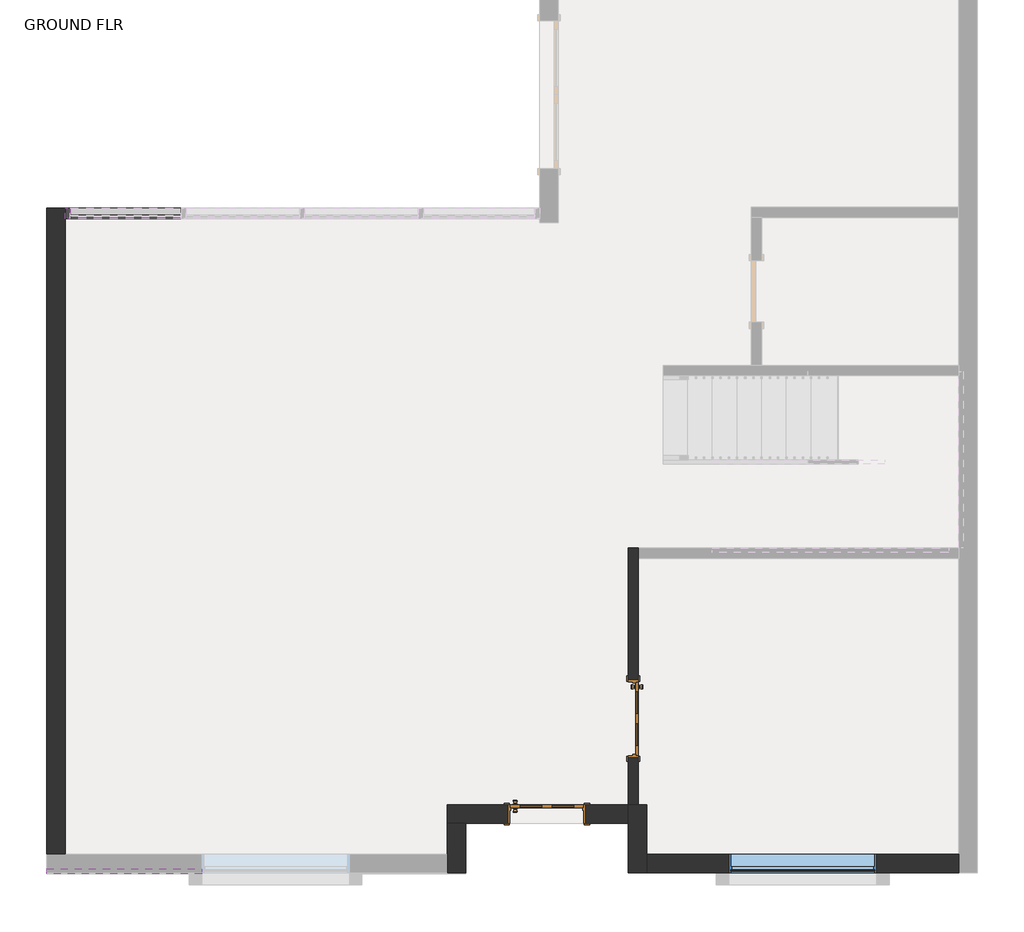
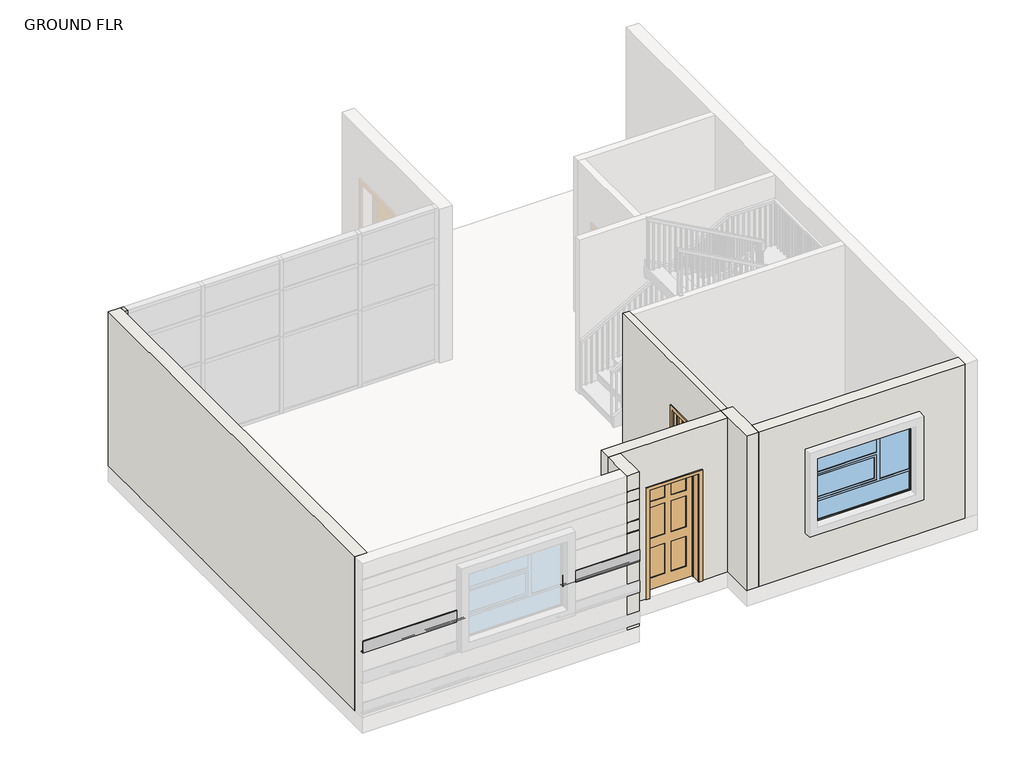
# One storey, part 2 of 4: 6 walls, 4 members, 2 doors, 1 proxy, 1 window.
"""IFC4 building model written with IfcOpenShell, lengths in millimetres."""

from ifc_helpers import new_model, si_unit, point, frame, frame_2d, origin, place, context, project, spatial, polyline, circle_curve, trimmed, segment, composite_curve, outline, extrude, faceted_brep, transform, mapped, element, save
from ifc_brep_helpers import plane_surface, cylinder_surface, revolved_surface, advanced_brep
from components import door_03e3dfb5, door_d86b6c54, member_bb3ab01a, member_47bfaf8a, member_4491d118, member_73c23c35, window_dd9b4f56

model = new_model("IFC4")

# Units and contexts
model_context = context("Model", 3, world=origin())
ifc_project = project(units=[si_unit("LENGTHUNIT", "METRE", prefix="MILLI")], contexts=[model_context])

# Site, building, storey
site = spatial("IfcSite", under=ifc_project)
building = spatial("IfcBuilding", under=site)
storey = spatial("IfcBuildingStorey", under=building, Name="GROUND FLR", Elevation=304.8)

# Proxy
placement = place(None, origin())
element("IfcBuildingElementProxy", 1, Name="Reveal", ObjectType="Reveal", at=placement, inside=storey, context=model_context, shape_type="SweptSolid", body=[
    extrude(outline(composite_curve([segment(polyline([(-2464.7620789, 1824.113469), (-2401.5160789, 1824.113469), (-2401.5160789, 1822.7337932)]), True, "CONTINUOUS"), segment(trimmed(circle_curve(frame_2d((-2406.7611789, 1822.7337932)), 5.2451), [point((-2401.5160789, 1822.7337932))], [point((-2405.8988881, 1817.5600587))], False, "CARTESIAN"), True, "CONTINUOUS"), segment(polyline([(-2405.8988881, 1817.5600587), (-2429.5195789, 1813.623269), (-2448.7574605, 1810.416949)]), True, "CONTINUOUS"), segment(trimmed(circle_curve(frame_2d((-2447.0328789, 1800.06948)), 10.4902), [point((-2448.7574605, 1810.416949))], [point((-2457.5230789, 1800.06948))], True, "CARTESIAN"), True, "CONTINUOUS"), segment(polyline([(-2457.5230789, 1800.06948), (-2457.5230789, 1619.557458)]), True, "CONTINUOUS"), segment(trimmed(circle_curve(frame_2d((-2447.0328789, 1619.557458)), 10.4902), [point((-2457.5230789, 1619.557458))], [point((-2448.7574605, 1609.209989))], True, "CARTESIAN"), True, "CONTINUOUS"), segment(polyline([(-2448.7574605, 1609.209989), (-2429.5195789, 1606.003669), (-2405.8988881, 1602.0668793)]), True, "CONTINUOUS"), segment(trimmed(circle_curve(frame_2d((-2406.7611789, 1596.8931449)), 5.2451), [point((-2405.8988881, 1602.0668793))], [point((-2401.5160789, 1596.8931449))], False, "CARTESIAN"), True, "CONTINUOUS"), segment(polyline([(-2401.5160789, 1596.8931449), (-2401.5160789, 1595.513469), (-2464.7620789, 1595.513469), (-2464.7620789, 1824.113469)]), True, "CONTINUOUS")], self_intersect=False)), frame((-2097.5328791, 0.0, 0.0), z_axis=(1.0, 0.0, 0.0), x_axis=(0.0, 1.0, 0.0)), (0.0, 0.0, 1.0), 1435.1),
    extrude(outline(composite_curve([segment(polyline([(-2464.7620789, 1824.113469), (-2401.5160789, 1824.113469), (-2401.5160789, 1822.7337932)]), True, "CONTINUOUS"), segment(trimmed(circle_curve(frame_2d((-2406.7611789, 1822.7337932)), 5.2451), [point((-2401.5160789, 1822.7337932))], [point((-2405.8988881, 1817.5600587))], False, "CARTESIAN"), True, "CONTINUOUS"), segment(polyline([(-2405.8988881, 1817.5600587), (-2429.5195789, 1813.623269), (-2448.7574605, 1810.416949)]), True, "CONTINUOUS"), segment(trimmed(circle_curve(frame_2d((-2447.0328789, 1800.06948)), 10.4902), [point((-2448.7574605, 1810.416949))], [point((-2457.5230789, 1800.06948))], True, "CARTESIAN"), True, "CONTINUOUS"), segment(polyline([(-2457.5230789, 1800.06948), (-2457.5230789, 1619.557458)]), True, "CONTINUOUS"), segment(trimmed(circle_curve(frame_2d((-2447.0328789, 1619.557458)), 10.4902), [point((-2457.5230789, 1619.557458))], [point((-2448.7574605, 1609.209989))], True, "CARTESIAN"), True, "CONTINUOUS"), segment(polyline([(-2448.7574605, 1609.209989), (-2429.5195789, 1606.003669), (-2405.8988881, 1602.0668793)]), True, "CONTINUOUS"), segment(trimmed(circle_curve(frame_2d((-2406.7611789, 1596.8931449)), 5.2451), [point((-2405.8988881, 1602.0668793))], [point((-2401.5160789, 1596.8931449))], False, "CARTESIAN"), True, "CONTINUOUS"), segment(polyline([(-2401.5160789, 1596.8931449), (-2401.5160789, 1595.513469), (-2464.7620789, 1595.513469), (-2464.7620789, 1824.113469)]), True, "CONTINUOUS")], self_intersect=False)), frame((-5844.0328791, 0.0, 0.0), z_axis=(1.0, 0.0, 0.0), x_axis=(0.0, 1.0, 0.0)), (0.0, 0.0, 1.0), 1917.7),
])

# Doors
door_shape = door_03e3dfb5(model_context)
element("IfcDoor", 2, ObjectType="Door-Interior-Single-6_Panel-Wood : 36\" x 84\"", at=placement, inside=storey, context=model_context, shape_type="MappedRepresentation", body=[
    mapped(door_shape, transform((1410.8421209, -544.8776789, 304.8), x_axis=(0.0, -1.0, 0.0), y_axis=(1.0, 0.0, 0.0), z_axis=(0.0, 0.0, 1.0))),
])
door_2_shape = door_d86b6c54(model_context)
element("IfcDoor", 3, ObjectType="Door-Interior-Single-6_Panel-Wood : 36\" x 84\"", at=placement, inside=storey, context=model_context, shape_type="MappedRepresentation", body=[
    mapped(door_2_shape, transform((340.8671209, -1722.8026789, 304.8), x_axis=(1.0, 0.0, 0.0), y_axis=(0.0, 1.0, 0.0), z_axis=(0.0, 0.0, 1.0))),
])

# Members
member_shape = member_bb3ab01a(model_context)
element("IfcMember", 4, ObjectType="Rectangular Mullion : 2.5\" x 5\" rectangular", at=placement, inside=storey, context=model_context, shape_type="MappedRepresentation", body=[
    mapped(member_shape, transform((-5551.9328791, 5703.5223211, 304.8), x_axis=(0.0, 0.0, -1.0), y_axis=(0.0, -1.0, 0.0), z_axis=(-1.0, 0.0, 0.0))),
])
member_2_shape = member_47bfaf8a(model_context)
element("IfcMember", 5, ObjectType="Rectangular Mullion : 2.5\" x 5\" rectangular", at=placement, inside=storey, context=model_context, shape_type="MappedRepresentation", body=[
    mapped(member_2_shape, transform((-5615.4328791, 5703.5223211, 3352.8), x_axis=(-1.0, 0.0, 0.0), y_axis=(0.0, -1.0, 0.0), z_axis=(0.0, 0.0, 1.0))),
])
member_3_shape = member_4491d118(model_context)
element("IfcMember", 6, ObjectType="Rectangular Mullion : 2.5\" x 5\" rectangular", at=placement, inside=storey, context=model_context, shape_type="MappedRepresentation", body=[
    mapped(member_3_shape, transform((-5615.4328791, 5703.5223211, 1828.8), x_axis=(-1.0, 0.0, 0.0), y_axis=(0.0, -1.0, 0.0), z_axis=(0.0, 0.0, 1.0))),
])
member_4_shape = member_73c23c35(model_context)
element("IfcMember", 7, ObjectType="Rectangular Mullion : 2.5\" x 5\" rectangular", at=placement, inside=storey, context=model_context, shape_type="MappedRepresentation", body=[
    mapped(member_4_shape, transform((-5615.4328791, 5703.5223211, 2743.2), x_axis=(-1.0, 0.0, 0.0), y_axis=(0.0, -1.0, 0.0), z_axis=(0.0, 0.0, 1.0))),
])

# Walls
element("IfcWall", 8, ObjectType="INNER WALL 5\"", at=placement, inside=storey, context=model_context, shape_type="Brep", body=[
    faceted_brep([(1471.1671209, 1563.3223211, 3352.8), (1471.1671209, 1436.3223211, 3352.8), (1471.1671209, -1611.6776789, 3352.8), (1471.1671209, -1611.6776789, 304.8), (1471.1671209, -1027.4776789, 304.8), (1471.1671209, -1027.4776789, 2463.8), (1471.1671209, -62.2776789, 2463.8), (1471.1671209, -62.2776789, 304.8), (1471.1671209, 1436.3223211, 304.8), (1471.1671209, 1563.3223211, 304.8), (1344.1671209, -1611.6776789, 3352.8), (1344.1671209, 1563.3223211, 3352.8), (1344.1671209, 1563.3223211, 304.8), (1344.1671209, -62.2776789, 304.8), (1344.1671209, -62.2776789, 2463.8), (1344.1671209, -1027.4776789, 2463.8), (1344.1671209, -1027.4776789, 304.8), (1344.1671209, -1611.6776789, 304.8)], [[[0, 1, 2, 3, 4, 5, 6, 7, 8, 9]], [[10, 11, 12, 13, 14, 15, 16, 17]], [[3, 17, 16, 4]], [[12, 9, 8, 7, 13]], [[2, 1, 0, 11, 10]], [[3, 2, 10, 17]], [[0, 9, 12, 11]], [[15, 5, 4, 16]], [[5, 15, 14, 6]], [[6, 14, 13, 7]]]),
])
element("IfcWall", 9, ObjectType="OUTER WALL 9\"", at=placement, inside=storey, context=model_context, shape_type="SweptSolid", body=[
    extrude(outline(polyline([(304.8, 5433.5671209), (3352.8, 5433.5671209), (3352.8, 1572.7671209), (304.8, 1572.7671209), (304.8, 5433.5671209)]), holes=[polyline([(2565.4, 2588.7671209), (2565.4, 4417.5671209), (1219.2, 4417.5671209), (1219.2, 2588.7671209), (2565.4, 2588.7671209)])]), frame((0.0, -2449.8776789, 0.0), z_axis=(0.0, 1.0, 0.0), x_axis=(0.0, 0.0, 1.0)), (0.0, 0.0, 1.0), 228.6),
])
element("IfcWall", 10, ObjectType="OUTER WALL 9\"", at=placement, inside=storey, context=model_context, shape_type="Brep", body=[
    faceted_brep([(1572.7671209, -2449.8776789, 304.8), (1572.7671209, -2221.2776789, 304.8), (1572.7671209, -1611.6776789, 304.8), (1572.7671209, -1611.6776789, 3352.8), (1572.7671209, -2221.2776789, 3352.8), (1572.7671209, -2449.8776789, 3352.8), (1344.1671209, -2449.8776789, 304.8), (1344.1671209, -2449.8776789, 3352.8), (1344.1671209, -1840.2776789, 3352.8), (1344.1671209, -1611.6776789, 3352.8), (1344.1671209, -1611.6776789, 304.8), (1344.1671209, -1840.2776789, 304.8), (1471.1671209, -1611.6776789, 304.8), (1471.1671209, -1611.6776789, 3352.8)], [[[0, 1, 2, 3, 4, 5]], [[6, 7, 8, 9, 10, 11]], [[2, 1, 0, 6, 11, 10, 12]], [[5, 4, 3, 13, 9, 8, 7]], [[0, 5, 7, 6]], [[3, 2, 12, 10, 9, 13]]]),
])
element("IfcWall", 11, ObjectType="OUTER WALL 9\"", at=placement, inside=storey, context=model_context, shape_type="Brep", body=[
    faceted_brep([(-891.0328791, -1611.6776789, 3352.8), (1344.1671209, -1611.6776789, 3352.8), (1344.1671209, -1611.6776789, 304.8), (823.4671209, -1611.6776789, 304.8), (823.4671209, -1611.6776789, 2463.8), (-141.7328791, -1611.6776789, 2463.8), (-141.7328791, -1611.6776789, 304.8), (-891.0328791, -1611.6776789, 304.8), (1344.1671209, -1840.2776789, 3352.8), (-662.4328791, -1840.2776789, 3352.8), (-891.0328791, -1840.2776789, 3352.8), (-891.0328791, -1840.2776789, 304.8), (-662.4328791, -1840.2776789, 304.8), (-141.7328791, -1840.2776789, 304.8), (-141.7328791, -1840.2776789, 2463.8), (823.4671209, -1840.2776789, 2463.8), (823.4671209, -1840.2776789, 304.8), (1344.1671209, -1840.2776789, 304.8)], [[[0, 1, 2, 3, 4, 5, 6, 7]], [[8, 9, 10, 11, 12, 13, 14, 15, 16, 17]], [[2, 17, 16, 3]], [[11, 7, 6, 13, 12]], [[1, 0, 10, 9, 8]], [[2, 1, 8, 17]], [[0, 7, 11, 10]], [[15, 4, 3, 16]], [[4, 15, 14, 5]], [[5, 14, 13, 6]]]),
])
element("IfcWall", 12, ObjectType="OUTER WALL 9\"", at=placement, inside=storey, context=model_context, shape_type="AdvancedBrep", body=[
    advanced_brep(
    [(-891.0328791, -1840.2776789, 304.8), (-891.0328791, -2221.2776789, 304.8), (-891.0328791, -2449.8776789, 304.8), (-891.0328791, -2449.8776789, 376.313469), (-891.0328791, -2401.5160789, 376.313469), (-891.0328791, -2401.5160789, 377.6931449), (-891.0328791, -2405.8988881, 382.8668793), (-891.0328791, -2429.5195789, 386.803669), (-891.0328791, -2448.7574605, 390.009989), (-891.0328791, -2449.8776789, 390.260359), (-891.0328791, -2449.8776789, 590.9665791), (-891.0328791, -2448.7574605, 591.216949), (-891.0328791, -2429.5195789, 594.423269), (-891.0328791, -2405.8988881, 598.3600587), (-891.0328791, -2401.5160789, 603.5337932), (-891.0328791, -2401.5160789, 604.913469), (-891.0328791, -2449.8776789, 604.913469), (-891.0328791, -2449.8776789, 985.913469), (-891.0328791, -2401.5160789, 985.913469), (-891.0328791, -2401.5160789, 987.2931449), (-891.0328791, -2405.8988881, 992.4668793), (-891.0328791, -2429.5195789, 996.403669), (-891.0328791, -2448.7574605, 999.609989), (-891.0328791, -2449.8776789, 999.860359), (-891.0328791, -2449.8776789, 1200.5665791), (-891.0328791, -2448.7574605, 1200.816949), (-891.0328791, -2429.5195789, 1204.023269), (-891.0328791, -2405.8988881, 1207.9600587), (-891.0328791, -2401.5160789, 1213.1337932), (-891.0328791, -2401.5160789, 1214.513469), (-891.0328791, -2449.8776789, 1214.513469), (-891.0328791, -2449.8776789, 1595.513469), (-891.0328791, -2401.5160789, 1595.513469), (-891.0328791, -2401.5160789, 1596.8931449), (-891.0328791, -2405.8988881, 1602.0668793), (-891.0328791, -2429.5195789, 1606.003669), (-891.0328791, -2448.7574605, 1609.209989), (-891.0328791, -2449.8776789, 1609.460359), (-891.0328791, -2449.8776789, 1810.1665791), (-891.0328791, -2448.7574605, 1810.416949), (-891.0328791, -2429.5195789, 1813.623269), (-891.0328791, -2405.8988881, 1817.5600587), (-891.0328791, -2401.5160789, 1822.7337932), (-891.0328791, -2401.5160789, 1824.113469), (-891.0328791, -2449.8776789, 1824.113469), (-891.0328791, -2449.8776789, 2205.113469), (-891.0328791, -2401.5160789, 2205.113469), (-891.0328791, -2401.5160789, 2206.4931449), (-891.0328791, -2405.8988881, 2211.6668793), (-891.0328791, -2429.5195789, 2215.603669), (-891.0328791, -2448.7574605, 2218.809989), (-891.0328791, -2449.8776789, 2219.060359), (-891.0328791, -2449.8776789, 2419.7665791), (-891.0328791, -2448.7574605, 2420.016949), (-891.0328791, -2429.5195789, 2423.223269), (-891.0328791, -2405.8988881, 2427.1600587), (-891.0328791, -2401.5160789, 2432.3337932), (-891.0328791, -2401.5160789, 2433.713469), (-891.0328791, -2449.8776789, 2433.713469), (-891.0328791, -2449.8776789, 2814.713469), (-891.0328791, -2401.5160789, 2814.713469), (-891.0328791, -2401.5160789, 2816.0931449), (-891.0328791, -2405.8988881, 2821.2668793), (-891.0328791, -2429.5195789, 2825.203669), (-891.0328791, -2448.7574605, 2828.409989), (-891.0328791, -2449.8776789, 2828.660359), (-891.0328791, -2449.8776789, 3029.3665791), (-891.0328791, -2448.7574605, 3029.616949), (-891.0328791, -2429.5195789, 3032.823269), (-891.0328791, -2405.8988881, 3036.7600587), (-891.0328791, -2401.5160789, 3041.9337932), (-891.0328791, -2401.5160789, 3043.313469), (-891.0328791, -2449.8776789, 3043.313469), (-891.0328791, -2449.8776789, 3352.8), (-891.0328791, -2221.2776789, 3352.8), (-891.0328791, -1840.2776789, 3352.8), (-662.4328791, -2449.8776789, 304.8), (-662.4328791, -1840.2776789, 304.8), (-662.4328791, -1840.2776789, 3352.8), (-662.4328791, -2449.8776789, 3352.8), (-662.4328791, -2449.8776789, 3043.313469), (-662.4328791, -2401.5160789, 3043.313469), (-662.4328791, -2401.5160789, 3041.9337932), (-662.4328791, -2405.8988881, 3036.7600587), (-662.4328791, -2429.5195789, 3032.823269), (-662.4328791, -2448.7574605, 3029.616949), (-662.4328791, -2449.8776789, 3029.3665791), (-662.4328791, -2449.8776789, 2828.660359), (-662.4328791, -2448.7574605, 2828.409989), (-662.4328791, -2429.5195789, 2825.203669), (-662.4328791, -2405.8988881, 2821.2668793), (-662.4328791, -2401.5160789, 2816.0931449), (-662.4328791, -2401.5160789, 2814.713469), (-662.4328791, -2449.8776789, 2814.713469), (-662.4328791, -2449.8776789, 2433.713469), (-662.4328791, -2401.5160789, 2433.713469), (-662.4328791, -2401.5160789, 2432.3337932), (-662.4328791, -2405.8988881, 2427.1600587), (-662.4328791, -2429.5195789, 2423.223269), (-662.4328791, -2448.7574605, 2420.016949), (-662.4328791, -2449.8776789, 2419.7665791), (-662.4328791, -2449.8776789, 2219.060359), (-662.4328791, -2448.7574605, 2218.809989), (-662.4328791, -2429.5195789, 2215.603669), (-662.4328791, -2405.8988881, 2211.6668793), (-662.4328791, -2401.5160789, 2206.4931449), (-662.4328791, -2401.5160789, 2205.113469), (-662.4328791, -2449.8776789, 2205.113469), (-662.4328791, -2449.8776789, 1824.113469), (-662.4328791, -2401.5160789, 1824.113469), (-662.4328791, -2401.5160789, 1822.7337932), (-662.4328791, -2405.8988881, 1817.5600587), (-662.4328791, -2429.5195789, 1813.623269), (-662.4328791, -2448.7574605, 1810.416949), (-662.4328791, -2449.8776789, 1810.1665791), (-662.4328791, -2449.8776789, 1609.460359), (-662.4328791, -2448.7574605, 1609.209989), (-662.4328791, -2429.5195789, 1606.003669), (-662.4328791, -2405.8988881, 1602.0668793), (-662.4328791, -2401.5160789, 1596.8931449), (-662.4328791, -2401.5160789, 1595.513469), (-662.4328791, -2449.8776789, 1595.513469), (-662.4328791, -2449.8776789, 1214.513469), (-662.4328791, -2401.5160789, 1214.513469), (-662.4328791, -2401.5160789, 1213.1337932), (-662.4328791, -2405.8988881, 1207.9600587), (-662.4328791, -2429.5195789, 1204.023269), (-662.4328791, -2448.7574605, 1200.816949), (-662.4328791, -2449.8776789, 1200.5665791), (-662.4328791, -2449.8776789, 999.860359), (-662.4328791, -2448.7574605, 999.609989), (-662.4328791, -2429.5195789, 996.403669), (-662.4328791, -2405.8988881, 992.4668793), (-662.4328791, -2401.5160789, 987.2931449), (-662.4328791, -2401.5160789, 985.913469), (-662.4328791, -2449.8776789, 985.913469), (-662.4328791, -2449.8776789, 604.913469), (-662.4328791, -2401.5160789, 604.913469), (-662.4328791, -2401.5160789, 603.5337932), (-662.4328791, -2405.8988881, 598.3600587), (-662.4328791, -2429.5195789, 594.423269), (-662.4328791, -2448.7574605, 591.216949), (-662.4328791, -2449.8776789, 590.9665791), (-662.4328791, -2449.8776789, 390.260359), (-662.4328791, -2448.7574605, 390.009989), (-662.4328791, -2429.5195789, 386.803669), (-662.4328791, -2405.8988881, 382.8668793), (-662.4328791, -2401.5160789, 377.6931449), (-662.4328791, -2401.5160789, 376.313469), (-662.4328791, -2449.8776789, 376.313469)],
    [
        (0, 1),
        (1, 2),
        (2, 3),
        (3, 4),
        (4, 5),
        (5, 6, circle_curve(frame((-891.0328791, -2406.7611789, 377.6931449), z_axis=(1.0, 0.0, 0.0), x_axis=(0.0, 1.0, 0.0)), 5.2451)),
        (6, 7),
        (7, 8),
        (8, 9, circle_curve(frame((-891.0328791, -2447.0328789, 400.357458), z_axis=(-1.0, 0.0, 0.0), x_axis=(0.0, 1.0, 0.0)), 10.4902)),
        (9, 10),
        (10, 11, circle_curve(frame((-891.0328791, -2447.0328789, 580.86948), z_axis=(-1.0, 0.0, 0.0), x_axis=(0.0, 1.0, 0.0)), 10.4902)),
        (11, 12),
        (12, 13),
        (13, 14, circle_curve(frame((-891.0328791, -2406.7611789, 603.5337932), z_axis=(1.0, 0.0, 0.0), x_axis=(0.0, 1.0, 0.0)), 5.2451)),
        (14, 15),
        (15, 16),
        (16, 17),
        (17, 18),
        (18, 19),
        (19, 20, circle_curve(frame((-891.0328791, -2406.7611789, 987.2931449), z_axis=(1.0, 0.0, 0.0), x_axis=(0.0, 1.0, 0.0)), 5.2451)),
        (20, 21),
        (21, 22),
        (22, 23, circle_curve(frame((-891.0328791, -2447.0328789, 1009.957458), z_axis=(-1.0, 0.0, 0.0), x_axis=(0.0, 1.0, 0.0)), 10.4902)),
        (23, 24),
        (24, 25, circle_curve(frame((-891.0328791, -2447.0328789, 1190.46948), z_axis=(-1.0, 0.0, 0.0), x_axis=(0.0, 1.0, 0.0)), 10.4902)),
        (25, 26),
        (26, 27),
        (27, 28, circle_curve(frame((-891.0328791, -2406.7611789, 1213.1337932), z_axis=(1.0, 0.0, 0.0), x_axis=(0.0, 1.0, 0.0)), 5.2451)),
        (28, 29),
        (29, 30),
        (30, 31),
        (31, 32),
        (32, 33),
        (33, 34, circle_curve(frame((-891.0328791, -2406.7611789, 1596.8931449), z_axis=(1.0, 0.0, 0.0), x_axis=(0.0, 1.0, 0.0)), 5.2451)),
        (34, 35),
        (35, 36),
        (36, 37, circle_curve(frame((-891.0328791, -2447.0328789, 1619.557458), z_axis=(-1.0, 0.0, 0.0), x_axis=(0.0, 1.0, 0.0)), 10.4902)),
        (37, 38),
        (38, 39, circle_curve(frame((-891.0328791, -2447.0328789, 1800.06948), z_axis=(-1.0, 0.0, 0.0), x_axis=(0.0, 1.0, 0.0)), 10.4902)),
        (39, 40),
        (40, 41),
        (41, 42, circle_curve(frame((-891.0328791, -2406.7611789, 1822.7337932), z_axis=(1.0, 0.0, 0.0), x_axis=(0.0, 1.0, 0.0)), 5.2451)),
        (42, 43),
        (43, 44),
        (44, 45),
        (45, 46),
        (46, 47),
        (47, 48, circle_curve(frame((-891.0328791, -2406.7611789, 2206.4931449), z_axis=(1.0, 0.0, 0.0), x_axis=(0.0, 1.0, 0.0)), 5.2451)),
        (48, 49),
        (49, 50),
        (50, 51, circle_curve(frame((-891.0328791, -2447.0328789, 2229.157458), z_axis=(-1.0, 0.0, 0.0), x_axis=(0.0, 1.0, 0.0)), 10.4902)),
        (51, 52),
        (52, 53, circle_curve(frame((-891.0328791, -2447.0328789, 2409.66948), z_axis=(-1.0, 0.0, 0.0), x_axis=(0.0, 1.0, 0.0)), 10.4902)),
        (53, 54),
        (54, 55),
        (55, 56, circle_curve(frame((-891.0328791, -2406.7611789, 2432.3337932), z_axis=(1.0, 0.0, 0.0), x_axis=(0.0, 1.0, 0.0)), 5.2451)),
        (56, 57),
        (57, 58),
        (58, 59),
        (59, 60),
        (60, 61),
        (61, 62, circle_curve(frame((-891.0328791, -2406.7611789, 2816.0931449), z_axis=(1.0, 0.0, 0.0), x_axis=(0.0, 1.0, 0.0)), 5.2451)),
        (62, 63),
        (63, 64),
        (64, 65, circle_curve(frame((-891.0328791, -2447.0328789, 2838.757458), z_axis=(-1.0, 0.0, 0.0), x_axis=(0.0, 1.0, 0.0)), 10.4902)),
        (65, 66),
        (66, 67, circle_curve(frame((-891.0328791, -2447.0328789, 3019.26948), z_axis=(-1.0, 0.0, 0.0), x_axis=(0.0, 1.0, 0.0)), 10.4902)),
        (67, 68),
        (68, 69),
        (69, 70, circle_curve(frame((-891.0328791, -2406.7611789, 3041.9337932), z_axis=(1.0, 0.0, 0.0), x_axis=(0.0, 1.0, 0.0)), 5.2451)),
        (70, 71),
        (71, 72),
        (72, 73),
        (73, 74),
        (74, 75),
        (75, 0),
        (76, 77),
        (77, 78),
        (78, 79),
        (79, 80),
        (80, 81),
        (81, 82),
        (82, 83, circle_curve(frame((-662.4328791, -2406.7611789, 3041.9337932), z_axis=(-1.0, 0.0, 0.0), x_axis=(0.0, 1.0, 0.0)), 5.2451)),
        (83, 84),
        (84, 85),
        (85, 86, circle_curve(frame((-662.4328791, -2447.0328789, 3019.26948), z_axis=(1.0, 0.0, 0.0), x_axis=(0.0, 1.0, 0.0)), 10.4902)),
        (86, 87),
        (87, 88, circle_curve(frame((-662.4328791, -2447.0328789, 2838.757458), z_axis=(1.0, 0.0, 0.0), x_axis=(0.0, 1.0, 0.0)), 10.4902)),
        (88, 89),
        (89, 90),
        (90, 91, circle_curve(frame((-662.4328791, -2406.7611789, 2816.0931449), z_axis=(-1.0, 0.0, 0.0), x_axis=(0.0, 1.0, 0.0)), 5.2451)),
        (91, 92),
        (92, 93),
        (93, 94),
        (94, 95),
        (95, 96),
        (96, 97, circle_curve(frame((-662.4328791, -2406.7611789, 2432.3337932), z_axis=(-1.0, 0.0, 0.0), x_axis=(0.0, 1.0, 0.0)), 5.2451)),
        (97, 98),
        (98, 99),
        (99, 100, circle_curve(frame((-662.4328791, -2447.0328789, 2409.66948), z_axis=(1.0, 0.0, 0.0), x_axis=(0.0, 1.0, 0.0)), 10.4902)),
        (100, 101),
        (101, 102, circle_curve(frame((-662.4328791, -2447.0328789, 2229.157458), z_axis=(1.0, 0.0, 0.0), x_axis=(0.0, 1.0, 0.0)), 10.4902)),
        (102, 103),
        (103, 104),
        (104, 105, circle_curve(frame((-662.4328791, -2406.7611789, 2206.4931449), z_axis=(-1.0, 0.0, 0.0), x_axis=(0.0, 1.0, 0.0)), 5.2451)),
        (105, 106),
        (106, 107),
        (107, 108),
        (108, 109),
        (109, 110),
        (110, 111, circle_curve(frame((-662.4328791, -2406.7611789, 1822.7337932), z_axis=(-1.0, 0.0, 0.0), x_axis=(0.0, 1.0, 0.0)), 5.2451)),
        (111, 112),
        (112, 113),
        (113, 114, circle_curve(frame((-662.4328791, -2447.0328789, 1800.06948), z_axis=(1.0, 0.0, 0.0), x_axis=(0.0, 1.0, 0.0)), 10.4902)),
        (114, 115),
        (115, 116, circle_curve(frame((-662.4328791, -2447.0328789, 1619.557458), z_axis=(1.0, 0.0, 0.0), x_axis=(0.0, 1.0, 0.0)), 10.4902)),
        (116, 117),
        (117, 118),
        (118, 119, circle_curve(frame((-662.4328791, -2406.7611789, 1596.8931449), z_axis=(-1.0, 0.0, 0.0), x_axis=(0.0, 1.0, 0.0)), 5.2451)),
        (119, 120),
        (120, 121),
        (121, 122),
        (122, 123),
        (123, 124),
        (124, 125, circle_curve(frame((-662.4328791, -2406.7611789, 1213.1337932), z_axis=(-1.0, 0.0, 0.0), x_axis=(0.0, 1.0, 0.0)), 5.2451)),
        (125, 126),
        (126, 127),
        (127, 128, circle_curve(frame((-662.4328791, -2447.0328789, 1190.46948), z_axis=(1.0, 0.0, 0.0), x_axis=(0.0, 1.0, 0.0)), 10.4902)),
        (128, 129),
        (129, 130, circle_curve(frame((-662.4328791, -2447.0328789, 1009.957458), z_axis=(1.0, 0.0, 0.0), x_axis=(0.0, 1.0, 0.0)), 10.4902)),
        (130, 131),
        (131, 132),
        (132, 133, circle_curve(frame((-662.4328791, -2406.7611789, 987.2931449), z_axis=(-1.0, 0.0, 0.0), x_axis=(0.0, 1.0, 0.0)), 5.2451)),
        (133, 134),
        (134, 135),
        (135, 136),
        (136, 137),
        (137, 138),
        (138, 139, circle_curve(frame((-662.4328791, -2406.7611789, 603.5337932), z_axis=(-1.0, 0.0, 0.0), x_axis=(0.0, 1.0, 0.0)), 5.2451)),
        (139, 140),
        (140, 141),
        (141, 142, circle_curve(frame((-662.4328791, -2447.0328789, 580.86948), z_axis=(1.0, 0.0, 0.0), x_axis=(0.0, 1.0, 0.0)), 10.4902)),
        (142, 143),
        (143, 144, circle_curve(frame((-662.4328791, -2447.0328789, 400.357458), z_axis=(1.0, 0.0, 0.0), x_axis=(0.0, 1.0, 0.0)), 10.4902)),
        (144, 145),
        (145, 146),
        (146, 147, circle_curve(frame((-662.4328791, -2406.7611789, 377.6931449), z_axis=(-1.0, 0.0, 0.0), x_axis=(0.0, 1.0, 0.0)), 5.2451)),
        (147, 148),
        (148, 149),
        (149, 76),
        (0, 77),
        (76, 2),
        (73, 79),
        (78, 75),
        (149, 3),
        (72, 80),
        (142, 10),
        (9, 143),
        (16, 136),
        (135, 17),
        (30, 122),
        (121, 31),
        (23, 129),
        (128, 24),
        (93, 59),
        (58, 94),
        (65, 87),
        (86, 66),
        (107, 45),
        (44, 108),
        (51, 101),
        (100, 52),
        (37, 115),
        (114, 38),
        (141, 11),
        (140, 12),
        (139, 13),
        (138, 14),
        (137, 15),
        (8, 144),
        (7, 145),
        (146, 6),
        (5, 147),
        (148, 4),
        (134, 18),
        (133, 19),
        (132, 20),
        (131, 21),
        (130, 22),
        (127, 25),
        (126, 26),
        (125, 27),
        (124, 28),
        (123, 29),
        (92, 60),
        (91, 61),
        (90, 62),
        (89, 63),
        (88, 64),
        (85, 67),
        (84, 68),
        (83, 69),
        (82, 70),
        (81, 71),
        (106, 46),
        (105, 47),
        (104, 48),
        (103, 49),
        (102, 50),
        (99, 53),
        (98, 54),
        (97, 55),
        (96, 56),
        (95, 57),
        (120, 32),
        (119, 33),
        (118, 34),
        (117, 35),
        (116, 36),
        (113, 39),
        (112, 40),
        (111, 41),
        (110, 42),
        (109, 43),
    ],
    [
        plane_surface(frame((-891.0328791, -1840.2776789, 304.8), z_axis=(-1.0, 0.0, 0.0), x_axis=(0.0, -1.0, 0.0))),
        plane_surface(frame((-662.4328791, -1840.2776789, 304.8), z_axis=(1.0, 0.0, 0.0), x_axis=(0.0, 1.0, 0.0))),
        plane_surface(frame((-891.0328791, -1725.9776789, 304.8), z_axis=(0.0, 0.0, -1.0), x_axis=(1.0, 0.0, 0.0))),
        plane_surface(frame((-891.0328791, -2335.5776789, 3352.8), z_axis=(0.0, 0.0, 1.0), x_axis=(1.0, 0.0, 0.0))),
        plane_surface(frame((1344.1671209, -1840.2776789, 304.8), z_axis=(0.0, 1.0, 0.0), x_axis=(1.0, 0.0, 0.0))),
        plane_surface(frame((-662.4328791, -2449.8776789, 304.8), z_axis=(0.0, -1.0, 0.0), x_axis=(1.0, 0.0, 0.0))),
        cylinder_surface(frame((-662.4328791, -2447.0328789, 580.86948), z_axis=(-1.0, 0.0, 0.0), x_axis=(0.0, 1.0, 0.0)), 10.4902),
        plane_surface(frame((-662.4328791, -2448.7574605, 591.216949), z_axis=(0.0, -0.16439930721687146, 0.9863938705135048), x_axis=(-1.0, 0.0, 0.0))),
        plane_surface(frame((-662.4328791, -2429.5195789, 594.423269), z_axis=(0.0, -0.16439930721687082, 0.9863938705135049), x_axis=(-1.0, 0.0, 0.0))),
        revolved_surface(polyline([(-662.4328791, -2401.5160788999997, 603.5337932), (-891.0328791, -2401.5160788999997, 603.5337932)]), (-662.4328791, -2406.7611789, 603.5337932), (1.0, 0.0, 0.0)),
        plane_surface(frame((-662.4328791, -2401.5160789, 603.5337932), z_axis=(0.0, -1.0, 0.0), x_axis=(-1.0, 0.0, 0.0))),
        plane_surface(frame((-662.4328791, -2401.5160789, 604.913469), z_axis=(0.0, 0.0, -1.0), x_axis=(-1.0, 0.0, 0.0))),
        cylinder_surface(frame((-662.4328791, -2447.0328789, 400.357458), z_axis=(-1.0, 0.0, 0.0), x_axis=(0.0, 1.0, 0.0)), 10.4902),
        plane_surface(frame((-662.4328791, -2429.5195789, 386.803669), z_axis=(0.0, -0.1643993072168769, -0.9863938705135039), x_axis=(-1.0, 0.0, 0.0))),
        revolved_surface(polyline([(-662.4328791, -2401.5160788999997, 377.6931449), (-891.0328791, -2401.5160788999997, 377.6931449)]), (-662.4328791, -2406.7611789, 377.6931449), (1.0, 0.0, 0.0)),
        plane_surface(frame((-662.4328791, -2405.8988881, 382.8668793), z_axis=(0.0, -0.16439930721687793, -0.9863938705135037), x_axis=(-1.0, 0.0, 0.0))),
        plane_surface(frame((-662.4328791, -2464.7620789, 376.313469), z_axis=(0.0, 0.0, 1.0), x_axis=(-1.0, 0.0, 0.0))),
        plane_surface(frame((-662.4328791, -2401.5160789, 376.313469), z_axis=(0.0, -1.0, 0.0), x_axis=(-1.0, 0.0, 0.0))),
        plane_surface(frame((-662.4328791, -2464.7620789, 985.913469), z_axis=(0.0, 0.0, 1.0), x_axis=(-1.0, 0.0, 0.0))),
        plane_surface(frame((-662.4328791, -2401.5160789, 985.913469), z_axis=(0.0, -1.0, 0.0), x_axis=(-1.0, 0.0, 0.0))),
        revolved_surface(polyline([(-662.4328791, -2401.5160788999997, 987.2931449), (-891.0328791, -2401.5160788999997, 987.2931449)]), (-662.4328791, -2406.7611789, 987.2931449), (1.0, 0.0, 0.0)),
        plane_surface(frame((-662.4328791, -2405.8988881, 992.4668793), z_axis=(0.0, -0.16439930721687793, -0.9863938705135037), x_axis=(-1.0, 0.0, 0.0))),
        plane_surface(frame((-662.4328791, -2429.5195789, 996.403669), z_axis=(0.0, -0.1643993072168769, -0.9863938705135039), x_axis=(-1.0, 0.0, 0.0))),
        cylinder_surface(frame((-662.4328791, -2447.0328789, 1009.957458), z_axis=(-1.0, 0.0, 0.0), x_axis=(0.0, 1.0, 0.0)), 10.4902),
        cylinder_surface(frame((-662.4328791, -2447.0328789, 1190.46948), z_axis=(-1.0, 0.0, 0.0), x_axis=(0.0, 1.0, 0.0)), 10.4902),
        plane_surface(frame((-662.4328791, -2448.7574605, 1200.816949), z_axis=(0.0, -0.16439930721687146, 0.9863938705135048), x_axis=(-1.0, 0.0, 0.0))),
        plane_surface(frame((-662.4328791, -2429.5195789, 1204.023269), z_axis=(0.0, -0.16439930721687082, 0.9863938705135049), x_axis=(-1.0, 0.0, 0.0))),
        revolved_surface(polyline([(-662.4328791, -2401.5160788999997, 1213.1337932), (-891.0328791, -2401.5160788999997, 1213.1337932)]), (-662.4328791, -2406.7611789, 1213.1337932), (1.0, 0.0, 0.0)),
        plane_surface(frame((-662.4328791, -2401.5160789, 1213.1337932), z_axis=(0.0, -1.0, 0.0), x_axis=(-1.0, 0.0, 0.0))),
        plane_surface(frame((-662.4328791, -2401.5160789, 1214.513469), z_axis=(0.0, 0.0, -1.0), x_axis=(-1.0, 0.0, 0.0))),
        plane_surface(frame((-662.4328791, -2464.7620789, 2814.713469), z_axis=(0.0, 0.0, 1.0), x_axis=(-1.0, 0.0, 0.0))),
        plane_surface(frame((-662.4328791, -2401.5160789, 2814.713469), z_axis=(0.0, -1.0, 0.0), x_axis=(-1.0, 0.0, 0.0))),
        revolved_surface(polyline([(-662.4328791, -2401.5160788999997, 2816.0931449), (-891.0328791, -2401.5160788999997, 2816.0931449)]), (-662.4328791, -2406.7611789, 2816.0931449), (1.0, 0.0, 0.0)),
        plane_surface(frame((-662.4328791, -2405.8988881, 2821.2668793), z_axis=(0.0, -0.16439930721687793, -0.9863938705135037), x_axis=(-1.0, 0.0, 0.0))),
        plane_surface(frame((-662.4328791, -2429.5195789, 2825.203669), z_axis=(0.0, -0.1643993072168769, -0.9863938705135039), x_axis=(-1.0, 0.0, 0.0))),
        cylinder_surface(frame((-662.4328791, -2447.0328789, 2838.757458), z_axis=(-1.0, 0.0, 0.0), x_axis=(0.0, 1.0, 0.0)), 10.4902),
        cylinder_surface(frame((-662.4328791, -2447.0328789, 3019.26948), z_axis=(-1.0, 0.0, 0.0), x_axis=(0.0, 1.0, 0.0)), 10.4902),
        plane_surface(frame((-662.4328791, -2448.7574605, 3029.616949), z_axis=(0.0, -0.16439930721687146, 0.9863938705135048), x_axis=(-1.0, 0.0, 0.0))),
        plane_surface(frame((-662.4328791, -2429.5195789, 3032.823269), z_axis=(0.0, -0.16439930721687082, 0.9863938705135049), x_axis=(-1.0, 0.0, 0.0))),
        revolved_surface(polyline([(-662.4328791, -2401.5160788999997, 3041.9337932), (-891.0328791, -2401.5160788999997, 3041.9337932)]), (-662.4328791, -2406.7611789, 3041.9337932), (1.0, 0.0, 0.0)),
        plane_surface(frame((-662.4328791, -2401.5160789, 3041.9337932), z_axis=(0.0, -1.0, 0.0), x_axis=(-1.0, 0.0, 0.0))),
        plane_surface(frame((-662.4328791, -2401.5160789, 3043.313469), z_axis=(0.0, 0.0, -1.0), x_axis=(-1.0, 0.0, 0.0))),
        plane_surface(frame((-662.4328791, -2464.7620789, 2205.113469), z_axis=(0.0, 0.0, 1.0), x_axis=(-1.0, 0.0, 0.0))),
        plane_surface(frame((-662.4328791, -2401.5160789, 2205.113469), z_axis=(0.0, -1.0, 0.0), x_axis=(-1.0, 0.0, 0.0))),
        revolved_surface(polyline([(-662.4328791, -2401.5160788999997, 2206.4931449), (-891.0328791, -2401.5160788999997, 2206.4931449)]), (-662.4328791, -2406.7611789, 2206.4931449), (1.0, 0.0, 0.0)),
        plane_surface(frame((-662.4328791, -2405.8988881, 2211.6668793), z_axis=(0.0, -0.16439930721687793, -0.9863938705135037), x_axis=(-1.0, 0.0, 0.0))),
        plane_surface(frame((-662.4328791, -2429.5195789, 2215.603669), z_axis=(0.0, -0.1643993072168769, -0.9863938705135039), x_axis=(-1.0, 0.0, 0.0))),
        cylinder_surface(frame((-662.4328791, -2447.0328789, 2229.157458), z_axis=(-1.0, 0.0, 0.0), x_axis=(0.0, 1.0, 0.0)), 10.4902),
        cylinder_surface(frame((-662.4328791, -2447.0328789, 2409.66948), z_axis=(-1.0, 0.0, 0.0), x_axis=(0.0, 1.0, 0.0)), 10.4902),
        plane_surface(frame((-662.4328791, -2448.7574605, 2420.016949), z_axis=(0.0, -0.16439930721687146, 0.9863938705135048), x_axis=(-1.0, 0.0, 0.0))),
        plane_surface(frame((-662.4328791, -2429.5195789, 2423.223269), z_axis=(0.0, -0.16439930721687082, 0.9863938705135049), x_axis=(-1.0, 0.0, 0.0))),
        revolved_surface(polyline([(-662.4328791, -2401.5160788999997, 2432.3337932), (-891.0328791, -2401.5160788999997, 2432.3337932)]), (-662.4328791, -2406.7611789, 2432.3337932), (1.0, 0.0, 0.0)),
        plane_surface(frame((-662.4328791, -2401.5160789, 2432.3337932), z_axis=(0.0, -1.0, 0.0), x_axis=(-1.0, 0.0, 0.0))),
        plane_surface(frame((-662.4328791, -2401.5160789, 2433.713469), z_axis=(0.0, 0.0, -1.0), x_axis=(-1.0, 0.0, 0.0))),
        plane_surface(frame((-662.4328791, -2464.7620789, 1595.513469), z_axis=(0.0, 0.0, 1.0), x_axis=(-1.0, 0.0, 0.0))),
        plane_surface(frame((-662.4328791, -2401.5160789, 1595.513469), z_axis=(0.0, -1.0, 0.0), x_axis=(-1.0, 0.0, 0.0))),
        revolved_surface(polyline([(-662.4328791, -2401.5160788999997, 1596.8931449), (-891.0328791, -2401.5160788999997, 1596.8931449)]), (-662.4328791, -2406.7611789, 1596.8931449), (1.0, 0.0, 0.0)),
        plane_surface(frame((-662.4328791, -2405.8988881, 1602.0668793), z_axis=(0.0, -0.16439930721687793, -0.9863938705135037), x_axis=(-1.0, 0.0, 0.0))),
        plane_surface(frame((-662.4328791, -2429.5195789, 1606.003669), z_axis=(0.0, -0.1643993072168769, -0.9863938705135039), x_axis=(-1.0, 0.0, 0.0))),
        cylinder_surface(frame((-662.4328791, -2447.0328789, 1619.557458), z_axis=(-1.0, 0.0, 0.0), x_axis=(0.0, 1.0, 0.0)), 10.4902),
        cylinder_surface(frame((-662.4328791, -2447.0328789, 1800.06948), z_axis=(-1.0, 0.0, 0.0), x_axis=(0.0, 1.0, 0.0)), 10.4902),
        plane_surface(frame((-662.4328791, -2448.7574605, 1810.416949), z_axis=(0.0, -0.16439930721687146, 0.9863938705135048), x_axis=(-1.0, 0.0, 0.0))),
        plane_surface(frame((-662.4328791, -2429.5195789, 1813.623269), z_axis=(0.0, -0.16439930721687082, 0.9863938705135049), x_axis=(-1.0, 0.0, 0.0))),
        revolved_surface(polyline([(-662.4328791, -2401.5160788999997, 1822.7337932), (-891.0328791, -2401.5160788999997, 1822.7337932)]), (-662.4328791, -2406.7611789, 1822.7337932), (1.0, 0.0, 0.0)),
        plane_surface(frame((-662.4328791, -2401.5160789, 1822.7337932), z_axis=(0.0, -1.0, 0.0), x_axis=(-1.0, 0.0, 0.0))),
        plane_surface(frame((-662.4328791, -2401.5160789, 1824.113469), z_axis=(0.0, 0.0, -1.0), x_axis=(-1.0, 0.0, 0.0))),
    ],
    [
        (0, [[1, 2, 3, 4, 5, 6, 7, 8, 9, 10, 11, 12, 13, 14, 15, 16, 17, 18, 19, 20, 21, 22, 23, 24, 25, 26, 27, 28, 29, 30, 31, 32, 33, 34, 35, 36, 37, 38, 39, 40, 41, 42, 43, 44, 45, 46, 47, 48, 49, 50, 51, 52, 53, 54, 55, 56, 57, 58, 59, 60, 61, 62, 63, 64, 65, 66, 67, 68, 69, 70, 71, 72, 73, 74, 75, 76]]),
        (1, [[77, 78, 79, 80, 81, 82, 83, 84, 85, 86, 87, 88, 89, 90, 91, 92, 93, 94, 95, 96, 97, 98, 99, 100, 101, 102, 103, 104, 105, 106, 107, 108, 109, 110, 111, 112, 113, 114, 115, 116, 117, 118, 119, 120, 121, 122, 123, 124, 125, 126, 127, 128, 129, 130, 131, 132, 133, 134, 135, 136, 137, 138, 139, 140, 141, 142, 143, 144, 145, 146, 147, 148, 149, 150]]),
        (2, [[-2, -1, 151, -77, 152]]),
        (3, [[-75, -74, 153, -79, 154]]),
        (4, [[-76, -154, -78, -151]]),
        (5, [[-152, -150, 155, -3]]),
        (5, [[-153, -73, 156, -80]]),
        (5, [[157, -10, 158, -143]]),
        (5, [[159, -136, 160, -17]]),
        (5, [[161, -122, 162, -31]]),
        (5, [[-24, 163, -129, 164]]),
        (5, [[165, -59, 166, -94]]),
        (5, [[-66, 167, -87, 168]]),
        (5, [[169, -45, 170, -108]]),
        (5, [[-52, 171, -101, 172]]),
        (5, [[-38, 173, -115, 174]]),
        (6, [[175, -11, -157, -142]]),
        (7, [[-175, -141, 176, -12]]),
        (8, [[-176, -140, 177, -13]]),
        (9, [[-177, -139, 178, -14]]),
        (10, [[-178, -138, 179, -15]]),
        (11, [[-179, -137, -159, -16]]),
        (12, [[180, -144, -158, -9]]),
        (13, [[-180, -8, 181, -145]]),
        (14, [[182, -6, 183, -147]]),
        (15, [[-181, -7, -182, -146]]),
        (16, [[184, -4, -155, -149]]),
        (17, [[-183, -5, -184, -148]]),
        (18, [[185, -18, -160, -135]]),
        (19, [[-185, -134, 186, -19]]),
        (20, [[-186, -133, 187, -20]]),
        (21, [[-187, -132, 188, -21]]),
        (22, [[-188, -131, 189, -22]]),
        (23, [[-189, -130, -163, -23]]),
        (24, [[190, -25, -164, -128]]),
        (25, [[-190, -127, 191, -26]]),
        (26, [[-191, -126, 192, -27]]),
        (27, [[-192, -125, 193, -28]]),
        (28, [[-193, -124, 194, -29]]),
        (29, [[-194, -123, -161, -30]]),
        (30, [[195, -60, -165, -93]]),
        (31, [[-195, -92, 196, -61]]),
        (32, [[-196, -91, 197, -62]]),
        (33, [[-197, -90, 198, -63]]),
        (34, [[-198, -89, 199, -64]]),
        (35, [[-199, -88, -167, -65]]),
        (36, [[200, -67, -168, -86]]),
        (37, [[-200, -85, 201, -68]]),
        (38, [[-201, -84, 202, -69]]),
        (39, [[-202, -83, 203, -70]]),
        (40, [[-203, -82, 204, -71]]),
        (41, [[-204, -81, -156, -72]]),
        (42, [[205, -46, -169, -107]]),
        (43, [[-205, -106, 206, -47]]),
        (44, [[-206, -105, 207, -48]]),
        (45, [[-207, -104, 208, -49]]),
        (46, [[-208, -103, 209, -50]]),
        (47, [[-209, -102, -171, -51]]),
        (48, [[210, -53, -172, -100]]),
        (49, [[-210, -99, 211, -54]]),
        (50, [[-211, -98, 212, -55]]),
        (51, [[-212, -97, 213, -56]]),
        (52, [[-213, -96, 214, -57]]),
        (53, [[-214, -95, -166, -58]]),
        (54, [[215, -32, -162, -121]]),
        (55, [[-215, -120, 216, -33]]),
        (56, [[-216, -119, 217, -34]]),
        (57, [[-217, -118, 218, -35]]),
        (58, [[-218, -117, 219, -36]]),
        (59, [[-219, -116, -173, -37]]),
        (60, [[220, -39, -174, -114]]),
        (61, [[-220, -113, 221, -40]]),
        (62, [[-221, -112, 222, -41]]),
        (63, [[-222, -111, 223, -42]]),
        (64, [[-223, -110, 224, -43]]),
        (65, [[-224, -109, -170, -44]]),
    ],
),
])
element("IfcWall", 13, ObjectType="OUTER WALL 9\"", at=placement, inside=storey, context=model_context, shape_type="SweptSolid", body=[
    extrude(outline(polyline([(-5615.4328791, 5767.0223211), (-5615.4328791, -2221.2776789), (-5844.0328791, -2221.2776789), (-5844.0328791, 5767.0223211), (-5615.4328791, 5767.0223211)])), frame((0.0, 0.0, 304.8), z_axis=(0.0, 0.0, 1.0), x_axis=(1.0, 0.0, 0.0)), (0.0, 0.0, 1.0), 3048.0),
])

# Window
window_shape = window_dd9b4f56(model_context)
element("IfcWindow", 14, ObjectType="Window-Awning-Variable : 72\" x 53\" 2", at=placement, inside=storey, context=model_context, shape_type="MappedRepresentation", body=[
    mapped(window_shape, transform((3503.1671209, -2335.5776789, 304.8), x_axis=(-1.0, 0.0, 0.0), y_axis=(0.0, -1.0, 0.0), z_axis=(0.0, 0.0, 1.0))),
])

save(model, "model.ifc")

# Revit data of these elements
# Type "Door-Interior-Single-6_Panel-Wood : 36\" x 84\""
#   Type Mark = "8"
#   Assembly Code = "C1020300"
#   Analytic Construction = "Wooden"
#   Top Rail = 0' - 4 11/16"
#   Top Panel = 0' - 11"
#   Thickness = 0' - 1 3/8"
#   Thermal Resistance (R) = 2.5876 (h·ft²·°F)/BTU
#   Swing Angle [instance default] = 90.00°
#   Stiles = 0' - 4 3/4"
#   Rough Width = 3' - 2"
#   Rough Height = 7' - 1"
#   Mullion = 0' - 4 1/2"
#   Lock Rail = 0' - 7 1/2"
#   Intermediate Rail = 0' - 4 1/2"
#   Height = 7' - 0"
#   Width = 3' - 0"
#   Heat Transfer Coefficient (U) = 0.3865 BTU/(h·ft²·°F)
#   Bottom Rail = 0' - 9 1/8"
#   Trim Material = Cherry
#   Panel Material = Cherry
#   Frame Material = Cherry
#   Door Handle Material = Aluminum
#   Visual Light Transmittance = 0
#   Solar Heat Gain Coefficient = 0
#   Wall Closure = (empty or 0)
#   Function = (empty or 0)
# Type "Rectangular Mullion : 2.5\" x 5\" rectangular"
#   built-in parameter 1007304 = 0.416667 (stored number, unit not read)
#   built-in parameter 1007301 = 0.104167 (stored number, unit not read)
#   built-in parameter 1007300 = 0.104167 (stored number, unit not read)
# Type "INNER WALL 5\""
#   Assembly Code = "B2010"
#   Layers, outside or top first: 0' - 5" "OUTER WALL IVORY WHITE" (function 1)
# Type "OUTER WALL 9\""
#   Assembly Code = "B2010"
#   Layers, outside or top first: 0' - 9" "OUTER WALL IVORY WHITE" (function 1)
# Type "Window-Awning-Variable : 72\" x 53\" 2"
#   Type Mark = "21"
#   Fire Rating = "0.5h"
#   Assembly Code = "B2020100"
#   Analytic Construction = "Double glazing - domestic"
#   Window Inset [instance default] = 0' - 0 5/8"
#   Wall Thickness [instance default] = 0' - 6"
#   Visual Light Transmittance = 0.81
#   Transom Height Ratio = 0.3
#   Transom Height = 1' - 3.9"
#   Thermal Resistance (R) = 1.8146 (h·ft²·°F)/BTU
#   Solar Heat Gain Coefficient = 0.76
#   Rough Width = 6' - 0 1/2"
#   Rough Height = 4' - 5 1/2"
#   Opening Window Width = 4' - 0"
#   Opening Window Height = 1' - 9.2"
#   Heat Transfer Coefficient (U) = 0.5511 BTU/(h·ft²·°F)
#   Height = 4' - 5"
#   Frame Gap 3 [instance default] = 0' - 1 83/128"
#   Frame Gap 2 [instance default] = 0' - 0 5/8"
#   Frame Gap 1 = 0' - 1 51/128"
#   Fixed Window Width = 2' - 0"
#   Default Sill Height = 3' - 0"
#   Width = 6' - 0"
#   Frame Material = metal black
#   Glass Panel Material = Glass
#   Wall Closure = (empty or 0)
# Elements 2, 3 (IfcDoor, "Door-Interior-Single-6_Panel-Wood : 36\" x 84\"")
#   Swing Angle = 90.00°
#   Phase Created = New Construction
#   Materials on its faces: "Cherry", "Aluminum"
# Elements 4, 5, 6, 7 (IfcMember, "Rectangular Mullion : 2.5\" x 5\" rectangular")
#   Phase Created = New Construction
#   Materials on its faces: "metal black"
# Element 8 (IfcWall, "INNER WALL 5\"")
#   Top Offset = 0' - 0"
#   Base Offset = 0' - 0"
#   wall height = 10' - 0"
#   Phase Created = New Construction
#   Base Constraint = GROUND FLR
#   Top Constraint = FIRST FLOOR
#   Materials on its faces: "OUTER WALL IVORY WHITE"
# Elements 9, 10, 11, 12, 13 (IfcWall, "OUTER WALL 9\"")
#   Top Offset = 0' - 0"
#   Base Offset = 0' - 0"
#   wall height = 10' - 0"
#   Phase Created = New Construction
#   Base Constraint = GROUND FLR
#   Top Constraint = FIRST FLOOR
#   Materials on its faces: "OUTER WALL IVORY WHITE"
# Element 14 (IfcWindow, "Window-Awning-Variable : 72\" x 53\" 2")
#   Mark = "2"
#   Window Inset = 0' - 0 5/8"
#   Frame Gap 3 = 0' - 1 83/128"
#   Frame Gap 2 = 0' - 0 5/8"
#   Phase Created = New Construction
#   Materials on its faces: "Glass", "metal black"
# Materials
#   "Cherry": class "Wood", colour RGB 226 177 128, transparency 0, Description = "Prunus Serotina", Cost = 0
#   "Aluminum": class "Metal", colour RGB 247 247 247, transparency 0, Description = "Aluminum 6061", Cost = 0
#   "OUTER WALL IVORY WHITE": class "Generic", colour RGB 120 120 120, transparency 0, Cost = 0
#   "metal black": class "Generic", colour RGB 120 120 120, transparency 0, Cost = 0
#   "Glass": class "Glass", colour RGB 0 128 192, transparency 0.75, Description = "Soda Lime Glass", Cost = 0
